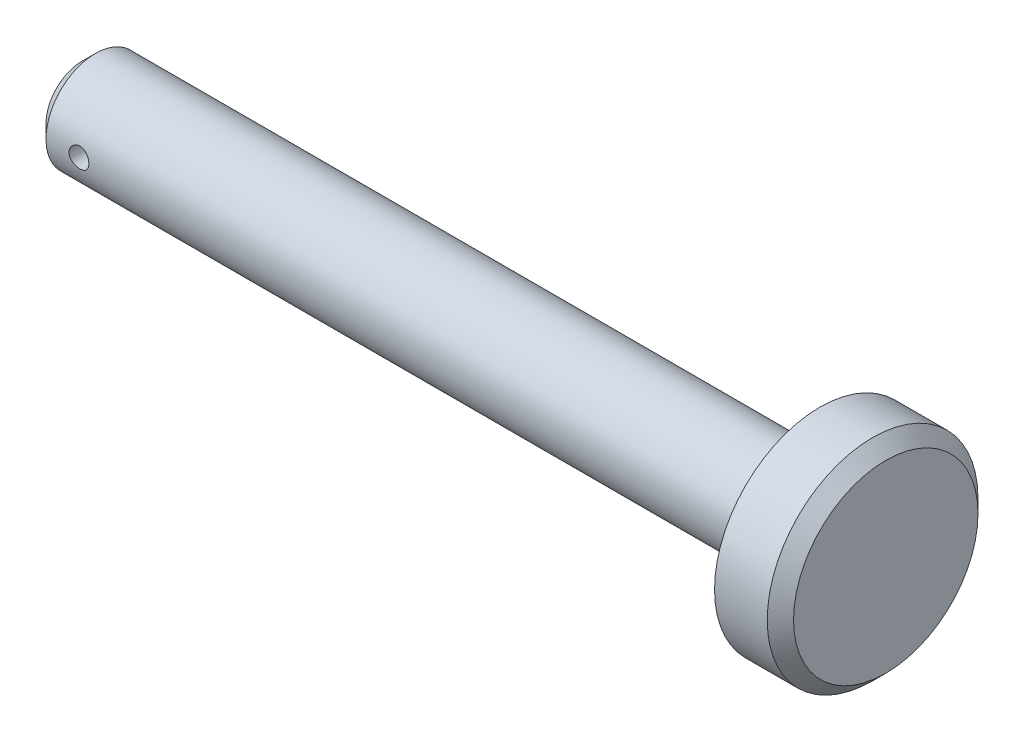
from build123d import *

# Parameters (mm, degrees)
CROSS_HOLE_3_DEPTH      = 125.080618954
CROSS_HOLE_3_DEPTH_BACK = 125.080618954
CROSS_HOLE_SKETCH_R     = 1.5
CHAMFER_2X45_SIZE       = 2


with BuildPart() as part:
    # Pin Profile Sketch → Pin Body (revolve)
    with BuildSketch(Plane.XY, mode=Mode.PRIVATE) as pin_body_sk:
        Polygon((0, -7.5), (112, -7.5), (112, -16), (122, -16), (122, 0), (0, 0), align=None)
    revolve(pin_body_sk.sketch.rotate(Axis((122, 0, 0), (-1, 0, 0)), 180), axis=Axis((122, 0, 0), (-1, 0, 0)))

    # Cross Hole Sketch → Cross Hole Ø3 (cut, two sides: drawn at the far end of the back side and taken through both)
    with BuildSketch(Plane.XY.offset(-CROSS_HOLE_3_DEPTH_BACK)):
        with Locations((7, 0)):
            Circle(CROSS_HOLE_SKETCH_R)
    extrude(amount=CROSS_HOLE_3_DEPTH + CROSS_HOLE_3_DEPTH_BACK, mode=Mode.SUBTRACT)

    # Chamfer 2x45°
    chamfer_2x45_edges = [part.edges().sort_by_distance(p)[0] for p in [
        (122, -16, 0),
        (0, -7.5, 0),
    ]]
    chamfer(chamfer_2x45_edges, length=CHAMFER_2X45_SIZE)


solid = part.part
